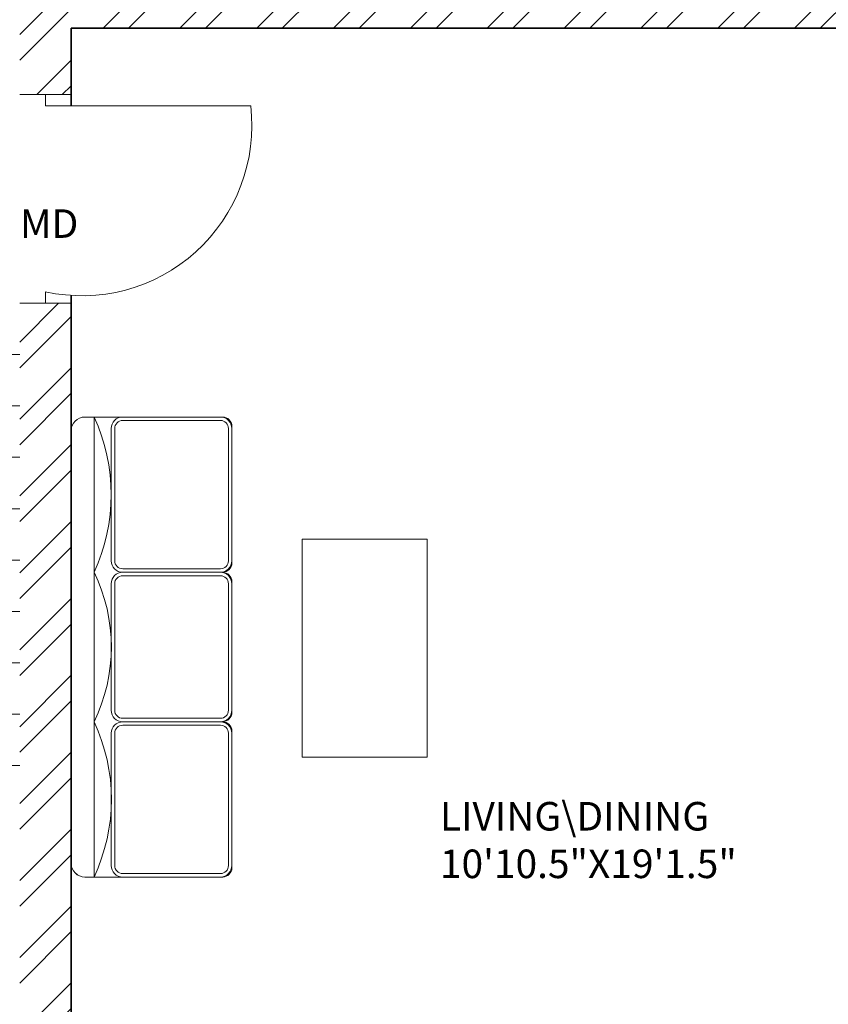
# Model space of a CAD drawing. Units: inches. Extents: x 2120 to 4013, y 1390 to 3019.
# Tile 23 of 59: x 2716 to 2857, y 1792 to 1964. Entities that reach past the tile are written whole.
import ezdxf

# ---------------------------------------------------------------- set-up
doc = ezdxf.new("R2010")
doc.units = ezdxf.units.IN
for name, color, linetype, lineweight in [('A-ANNO-TEXT', 7, 'Continuous', 18), ('A-AREA-IDEN', 7, 'Continuous', 18), ('A-DOOR', 3, 'Continuous', 18), ('A-FLOR-STRS', 7, 'Continuous', 18), ('A-FURN', 8, 'Continuous', 13), ('A-WALL', 7, 'Continuous', 35), ('A-WALL-PATT', 252, 'Continuous', 13)]:
    doc.layers.add(name, color=color, linetype=linetype, lineweight=lineweight)
doc.styles.get("Standard").update_dxf_attribs({"font": 'arial.ttf'})

# ---------------------------------------------------------------- blocks, each defined once
blk = doc.blocks.new('DOOR-SWING-36IN-109p07DEG')
for p, q in [((9, 36.56), (0, 36.56)), ((0, 36.56), (4.5, 36.56)), ((4.5, 36.56), (4.5, 34.56)), ((9, 36.56), (9, 36.56)), ((4.5, 34.56), (40.5, 34.56)), ((4.5, 0), (4.5, 2)), ((9, 0), (0, 0)), ((0, 0), (4.5, 0))]:
    blk.add_line(p, q)
blk.add_arc((10.9, 31.1), 29.8, 257.5927, 6.6652)
blk = doc.blocks.new('TABLE-COFFEE')
blk.add_lwpolyline([(0, 38.19), (21.88, 38.19), (21.88, 0), (0, 0)], close=True)
blk = doc.blocks.new('STAIR-DOGLEG-PLAN')
for p, q in [((60.72, 143.1), (60.72, 31.5)), ((39, 0), (39, 130.5)), ((78, 121.5), (0, 121.5)), ((78, 112.5), (0, 112.5)), ((78, 103.5), (0, 103.5)), ((78, 94.5), (0, 94.5)), ((78, 85.5), (0, 85.5)), ((78, 76.5), (0, 76.5)), ((78, 67.5), (0, 67.5)), ((18.01, 31.5), (18.01, 67.5)), ((78, 58.5), (0, 58.5)), ((78, 49.5), (0, 49.5)), ((60.72, 31.5), (18.01, 31.5)), ((60.72, 31.5), (18.01, 31.5))]:
    blk.add_line(p, q)

msp = doc.modelspace()

# ---------------------------------------------------------------- hatches: boundary and pattern name
at = {"layer": 'A-WALL-PATT'}
h = msp.add_hatch(dxfattribs=at)
h.set_pattern_fill('ANSI32', color=256)
h.paths.add_polyline_path([(2271.7331, 2343.531), (2283.3788, 2343.531), (2283.3788, 2348.031), (2283.3788, 2352.5306), (2262.7331, 2352.5306), (2262.7331, 2182.638), (2267.2331, 2182.638), (2271.7331, 2182.638), (2271.7331, 2219.031), (2391.7331, 2219.031), (2391.7331, 2214.189), (2393.9831, 2214.189), (2396.2331, 2214.189), (2396.2331, 2219.031), (2420.2331, 2219.031), (2420.2331, 2225.7535), (2417.2197, 2225.7535), (2415.7331, 2225.7535), (2415.7331, 2223.5306), (2271.7331, 2223.5306)])
h.paths.add_polyline_path([(2380.0942, 2352.5306), (2343.3788, 2352.5306), (2343.3788, 2343.531), (2363.2331, 2343.531), (2363.2331, 2288.8489), (2365.4831, 2288.8489), (2367.7331, 2288.8489), (2367.7331, 2343.531), (2380.0942, 2343.531)], flags=17)
h.paths.add_polyline_path([(2432.4339, 2352.5306), (2404.0943, 2352.5306), (2404.0943, 2343.531), (2415.7331, 2343.531), (2415.7331, 2264.0306), (2367.7331, 2264.0306), (2367.7331, 2266.4872), (2363.2331, 2266.4872), (2363.2331, 2259.531), (2367.7331, 2259.531), (2415.7331, 2259.531), (2415.7331, 2255.0658), (2420.2331, 2255.0658), (2420.2331, 2259.531), (2424.5717, 2259.531), (2424.5717, 2261.781), (2424.5717, 2264.0306), (2420.2331, 2264.0306), (2420.2331, 2343.531), (2432.4339, 2343.531)])
h.paths.add_polyline_path([(2508.9115, 2352.5306), (2456.4339, 2352.5306), (2456.4339, 2343.531), (2468.2331, 2343.531), (2468.2331, 2264.0306), (2448.0487, 2264.0306), (2448.0487, 2259.531), (2468.2331, 2259.531), (2468.2331, 2255.5496), (2472.7331, 2255.5496), (2472.7331, 2343.531), (2508.9115, 2343.531)])
h.paths.add_polyline_path([(2637.7331, 2352.5306), (2544.9116, 2352.5306), (2544.9116, 2343.531), (2589.7331, 2343.531), (2633.2331, 2343.531), (2637.7331, 2343.531)])
h.paths.add_polyline_path([(2594.2331, 2343.5306), (2589.7331, 2343.5306), (2589.7331, 2259.5306), (2589.7331, 2252.4915), (2591.9831, 2252.4915), (2594.2331, 2252.4915)])
h.paths.add_polyline_path([(2637.7331, 2223.5306), (2594.2331, 2223.5306), (2594.2331, 2230.1988), (2591.9831, 2230.1988), (2589.7331, 2230.1988), (2589.7331, 2223.5306), (2472.7331, 2223.5306), (2468.2331, 2223.5306), (2468.2331, 2219.031), (2628.7331, 2219.031), (2628.7331, 2138.031), (2637.7331, 2138.031)])
h.paths.add_polyline_path([(3822.6535, 2458.4402), (3874.9468, 2458.4402), (3874.9468, 2476.9866), (3822.6535, 2476.9866)], flags=9)
h.paths.add_polyline_path([(3834.6921, 2781.8174), (3935.9206, 2781.8174), (3935.9206, 2800.3638), (3834.6921, 2800.3638)], flags=9)
h.paths.add_polyline_path([(3832.2843, 2837.9683), (3884.5776, 2837.9683), (3884.5776, 2856.5146), (3832.2843, 2856.5146)], flags=9)
h.paths.add_polyline_path([(3830.9388, 2861.4782), (3956.8958, 2861.4782), (3956.8958, 2880.0245), (3830.9388, 2880.0245)], flags=9)
h.paths.add_polyline_path([(3870.6966, 2352.5752), (3887.9272, 2352.5752), (3887.9272, 2377.3037), (3870.6966, 2377.3037)], flags=9)
h.paths.add_polyline_path([(3289.2701, 2413.161), (3435.2223, 2413.161), (3435.2223, 2450.2538), (3289.2701, 2450.2538)], flags=9)
h.paths.add_polyline_path([(2487.6944, 2414.3601), (2637.8335, 2414.3601), (2637.8335, 2451.4528), (2487.6944, 2451.4528)], flags=9)
h.paths.add_polyline_path([(2567.3724, 1457.9199), (2815.296, 1457.9199), (2815.296, 1495.0127), (2567.3724, 1495.0127)], flags=9)
h.paths.add_polyline_path([(2655.3825, 2093.2363), (2685.9555, 2093.2363), (2685.9555, 2111.8937), (2655.3825, 2111.8937)], flags=9)
h.paths.add_polyline_path([(2543.9218, 1550.6671), (2587.8406, 1550.6671), (2587.8406, 1569.3244), (2543.9218, 1569.3244)], flags=9)
h.paths.add_polyline_path([(2905.1384, 1543.8113), (2949.0572, 1543.8113), (2949.0572, 1562.4686), (2905.1384, 1562.4686)], flags=9)
h.paths.add_polyline_path([(2736.4118, 1702.4736), (2784.2153, 1702.4736), (2784.2153, 1721.1309), (2736.4118, 1721.1309)], flags=9)
h.paths.add_polyline_path([(2912.8666, 1710.4168), (2951.707, 1710.4168), (2951.707, 1729.0741), (2912.8666, 1729.0741)], flags=9)
h.paths.add_polyline_path([(2923.5785, 1763.5038), (2959.7279, 1763.5038), (2959.7279, 1782.1611), (2923.5785, 1782.1611)], flags=9)
h.paths.add_polyline_path([(2925.2114, 1809.6137), (2967.1861, 1809.6137), (2967.1861, 1828.271), (2925.2114, 1828.271)], flags=9)
h.paths.add_polyline_path([(2996.2711, 1878.9003), (2996.2711, 1913.109), (2977.6138, 1913.109), (2977.6138, 1878.9003)], flags=9)
h.paths.add_polyline_path([(2883.0859, 1895.7192), (2927.1855, 1895.7192), (2927.1855, 1914.3766), (2883.0859, 1914.3766)], flags=9)
h.paths.add_polyline_path([(2787.3924, 1810.8013), (2841.0213, 1810.8013), (2841.0213, 1829.4587), (2787.3924, 1829.4587)], flags=9)
h.paths.add_polyline_path([(2775.6399, 2101.7395), (2829.2689, 2101.7395), (2829.2689, 2120.3968), (2775.6399, 2120.3968)], flags=9)
h.paths.add_polyline_path([(2913.0263, 2075.817), (2951.8667, 2075.817), (2951.8667, 2094.4744), (2913.0263, 2094.4744)], flags=9)
h.paths.add_polyline_path([(2929.966, 2133.3669), (2966.1154, 2133.3669), (2966.1154, 2152.0243), (2929.966, 2152.0243)], flags=9)
h.paths.add_polyline_path([(2932.7502, 2182.6088), (2968.8996, 2182.6088), (2968.8996, 2201.2662), (2932.7502, 2201.2662)], flags=9)
h.paths.add_polyline_path([(2996.0681, 2266.3173), (2996.0681, 2300.5261), (2977.4108, 2300.5261), (2977.4108, 2266.3173)], flags=9)
h.paths.add_polyline_path([(2885.1039, 2279.2186), (2929.2035, 2279.2186), (2929.2035, 2297.8759), (2885.1039, 2297.8759)], flags=9)
h.paths.add_polyline_path([(2735.7042, 2218.3197), (2783.5078, 2218.3197), (2783.5078, 2236.9771), (2735.7042, 2236.9771)], flags=9)
h.paths.add_polyline_path([(2635.6049, 2044.0085), (2648.9678, 2044.0085), (2648.9678, 2054.312), (2635.6049, 2054.312)], flags=9)
h.paths.add_polyline_path([(2714.0148, 1923.0473), (2727.3777, 1923.0473), (2727.3777, 1933.3508), (2714.0148, 1933.3508)], flags=9)
h.paths.add_polyline_path([(2709.0345, 1988.1628), (2722.3974, 1988.1628), (2722.3974, 1998.4663), (2709.0345, 1998.4663)], flags=9)
h.paths.add_polyline_path([(2592.8935, 1962.1763), (2606.2564, 1962.1763), (2606.2564, 1972.4799), (2592.8935, 1972.4799)], flags=9)
h.paths.add_polyline_path([(2618.3996, 1985.9724), (2644.1942, 1985.9724), (2644.1942, 1996.2759), (2618.3996, 1996.2759)], flags=9)
h.paths.add_polyline_path([(2601.279, 1920.5869), (2614.6419, 1920.5869), (2614.6419, 1930.8904), (2601.279, 1930.8904)], flags=9)
h.paths.add_polyline_path([(2692.3278, 1932.7645), (2704.5311, 1932.7645), (2704.5311, 1943.0681), (2692.3278, 1943.0681)], flags=9)
h.paths.add_polyline_path([(2311.122, 1672.7318), (2355.0408, 1672.7318), (2355.0408, 1691.3892), (2311.122, 1691.3892)], flags=9)
h.paths.add_polyline_path([(2456.2551, 1632.3198), (2492.4796, 1632.3198), (2492.4796, 1650.9772), (2456.2551, 1650.9772)], flags=9)
h.paths.add_polyline_path([(2401.0766, 1631.4793), (2437.301, 1631.4793), (2437.301, 1650.1367), (2401.0766, 1650.1367)], flags=9)
h.paths.add_polyline_path([(2546.7054, 1700.9235), (2594.509, 1700.9235), (2594.509, 1719.5809), (2546.7054, 1719.5809)], flags=9)
h.paths.add_polyline_path([(2445.4866, 1766.9937), (2497.5261, 1766.9937), (2497.5261, 1785.651), (2445.4866, 1785.651)], flags=9)
h.paths.add_polyline_path([(2287.9992, 1739.7675), (2326.8396, 1739.7675), (2326.8396, 1758.4248), (2287.9992, 1758.4248)], flags=9)
h.paths.add_polyline_path([(2458.5279, 1924.7607), (2510.5675, 1924.7607), (2510.5675, 1943.4181), (2458.5279, 1943.4181)], flags=9)
h.paths.add_polyline_path([(2309.2811, 1902.7642), (2345.4305, 1902.7642), (2345.4305, 1921.4215), (2309.2811, 1921.4215)], flags=9)
h.paths.add_polyline_path([(2490.7554, 2018.9392), (2530.7896, 2018.9392), (2530.7896, 2037.5965), (2490.7554, 2037.5965)], flags=9)
h.paths.add_polyline_path([(2402.143, 2024.7393), (2438.5414, 2024.7393), (2438.5414, 2043.3966), (2402.143, 2043.3966)], flags=9)
h.paths.add_polyline_path([(2287.856, 1931.7926), (2326.6964, 1931.7926), (2326.6964, 1950.4499), (2287.856, 1950.4499)], flags=9)
h.paths.add_polyline_path([(2281.7979, 2193.5771), (2320.6383, 2193.5771), (2320.6383, 2212.2344), (2281.7979, 2212.2344)], flags=25)
h.paths.add_polyline_path([(2484.0754, 2093.892), (2536.115, 2093.892), (2536.115, 2112.5494), (2484.0754, 2112.5494)], flags=9)
h.paths.add_polyline_path([(2624.7948, 2281.8639), (2624.7948, 2311.4137), (2606.1375, 2311.4137), (2606.1375, 2281.8639)], flags=9)
h.paths.add_polyline_path([(2507.5036, 2290.3639), (2541.934, 2290.3639), (2541.934, 2309.0212), (2507.5036, 2309.0212)], flags=9)
h.paths.add_polyline_path([(2423.1076, 2285.2202), (2459.332, 2285.2202), (2459.332, 2303.8776), (2423.1076, 2303.8776)], flags=9)
h.paths.add_polyline_path([(2374.5467, 2289.6272), (2410.7711, 2289.6272), (2410.7711, 2308.2846), (2374.5467, 2308.2846)], flags=25)
h.paths.add_polyline_path([(2277.4907, 2227.5651), (2316.3311, 2227.5651), (2316.3311, 2246.2224), (2277.4907, 2246.2224)], flags=25)
h.paths.add_polyline_path([(2655.3825, 2093.2367), (2685.9555, 2093.2367), (2685.9555, 2111.894), (2655.3825, 2111.894)], flags=9)
h.paths.add_polyline_path([(2543.9217, 1550.6674), (2587.8406, 1550.6674), (2587.8406, 1569.3247), (2543.9217, 1569.3247)], flags=9)
h.paths.add_polyline_path([(2905.1384, 1543.8116), (2949.0572, 1543.8116), (2949.0572, 1562.4689), (2905.1384, 1562.4689)], flags=9)
h.paths.add_polyline_path([(2736.4118, 1702.4739), (2784.2153, 1702.4739), (2784.2153, 1721.1312), (2736.4118, 1721.1312)], flags=9)
h.paths.add_polyline_path([(2912.8666, 1710.4171), (2951.707, 1710.4171), (2951.707, 1729.0744), (2912.8666, 1729.0744)], flags=9)
h.paths.add_polyline_path([(2923.5785, 1763.5041), (2959.7279, 1763.5041), (2959.7279, 1782.1614), (2923.5785, 1782.1614)], flags=9)
h.paths.add_polyline_path([(2925.2114, 1809.614), (2967.1861, 1809.614), (2967.1861, 1828.2713), (2925.2114, 1828.2713)], flags=9)
h.paths.add_polyline_path([(2996.2711, 1878.9006), (2996.2711, 1913.1094), (2977.6137, 1913.1094), (2977.6137, 1878.9006)], flags=9)
h.paths.add_polyline_path([(2883.0859, 1895.7195), (2927.1855, 1895.7195), (2927.1855, 1914.3769), (2883.0859, 1914.3769)], flags=9)
h.paths.add_polyline_path([(2787.3924, 1810.8016), (2841.0213, 1810.8016), (2841.0213, 1829.459), (2787.3924, 1829.459)], flags=9)
h.paths.add_polyline_path([(2775.6399, 2101.7398), (2829.2688, 2101.7398), (2829.2688, 2120.3971), (2775.6399, 2120.3971)], flags=9)
h.paths.add_polyline_path([(2913.0263, 2075.8173), (2951.8667, 2075.8173), (2951.8667, 2094.4747), (2913.0263, 2094.4747)], flags=9)
h.paths.add_polyline_path([(2929.966, 2133.3672), (2966.1154, 2133.3672), (2966.1154, 2152.0246), (2929.966, 2152.0246)], flags=9)
h.paths.add_polyline_path([(2932.7502, 2182.6091), (2968.8996, 2182.6091), (2968.8996, 2201.2665), (2932.7502, 2201.2665)], flags=9)
h.paths.add_polyline_path([(2996.0681, 2266.3176), (2996.0681, 2300.5264), (2977.4108, 2300.5264), (2977.4108, 2266.3176)], flags=9)
h.paths.add_polyline_path([(2885.1039, 2279.2189), (2929.2035, 2279.2189), (2929.2035, 2297.8762), (2885.1039, 2297.8762)], flags=9)
h.paths.add_polyline_path([(2735.7042, 2218.32), (2783.5078, 2218.32), (2783.5078, 2236.9774), (2735.7042, 2236.9774)], flags=9)
h.paths.add_polyline_path([(2635.6048, 2044.0088), (2648.9677, 2044.0088), (2648.9677, 2054.3123), (2635.6048, 2054.3123)], flags=9)
h.paths.add_polyline_path([(2714.0148, 1923.0476), (2727.3777, 1923.0476), (2727.3777, 1933.3511), (2714.0148, 1933.3511)], flags=9)
h.paths.add_polyline_path([(2709.0345, 1988.1631), (2722.3974, 1988.1631), (2722.3974, 1998.4666), (2709.0345, 1998.4666)], flags=9)
h.paths.add_polyline_path([(2592.8935, 1962.1766), (2606.2564, 1962.1766), (2606.2564, 1972.4802), (2592.8935, 1972.4802)], flags=9)
h.paths.add_polyline_path([(2618.3995, 1985.9727), (2644.1942, 1985.9727), (2644.1942, 1996.2762), (2618.3995, 1996.2762)], flags=9)
h.paths.add_polyline_path([(2601.279, 1920.5872), (2614.6419, 1920.5872), (2614.6419, 1930.8908), (2601.279, 1930.8908)], flags=9)
h.paths.add_polyline_path([(2692.3278, 1932.7648), (2704.5311, 1932.7648), (2704.5311, 1943.0684), (2692.3278, 1943.0684)], flags=9)
h.paths.add_polyline_path([(2311.122, 1672.7321), (2355.0408, 1672.7321), (2355.0408, 1691.3895), (2311.122, 1691.3895)], flags=9)
h.paths.add_polyline_path([(2456.2551, 1632.3201), (2492.4795, 1632.3201), (2492.4795, 1650.9775), (2456.2551, 1650.9775)], flags=9)
h.paths.add_polyline_path([(2401.0766, 1631.4796), (2437.301, 1631.4796), (2437.301, 1650.137), (2401.0766, 1650.137)], flags=9)
h.paths.add_polyline_path([(2546.7054, 1700.9238), (2594.509, 1700.9238), (2594.509, 1719.5812), (2546.7054, 1719.5812)], flags=9)
h.paths.add_polyline_path([(2445.4866, 1766.994), (2497.5261, 1766.994), (2497.5261, 1785.6513), (2445.4866, 1785.6513)], flags=9)
h.paths.add_polyline_path([(2287.9992, 1739.7678), (2326.8396, 1739.7678), (2326.8396, 1758.4251), (2287.9992, 1758.4251)], flags=9)
h.paths.add_polyline_path([(2458.5279, 1924.7611), (2510.5675, 1924.7611), (2510.5675, 1943.4184), (2458.5279, 1943.4184)], flags=9)
h.paths.add_polyline_path([(2309.2811, 1902.7645), (2345.4305, 1902.7645), (2345.4305, 1921.4218), (2309.2811, 1921.4218)], flags=9)
h.paths.add_polyline_path([(2490.7554, 2018.9395), (2530.7895, 2018.9395), (2530.7895, 2037.5968), (2490.7554, 2037.5968)], flags=9)
h.paths.add_polyline_path([(2402.143, 2024.7396), (2438.5413, 2024.7396), (2438.5413, 2043.3969), (2402.143, 2043.3969)], flags=9)
h.paths.add_polyline_path([(2287.856, 1931.7929), (2326.6964, 1931.7929), (2326.6964, 1950.4502), (2287.856, 1950.4502)], flags=9)
h.paths.add_polyline_path([(2281.7979, 2193.5774), (2320.6383, 2193.5774), (2320.6383, 2212.2347), (2281.7979, 2212.2347)], flags=25)
h.paths.add_polyline_path([(2484.0754, 2093.8924), (2536.115, 2093.8924), (2536.115, 2112.5497), (2484.0754, 2112.5497)], flags=9)
h.paths.add_polyline_path([(2624.7948, 2281.8642), (2624.7948, 2311.414), (2606.1374, 2311.414), (2606.1374, 2281.8642)], flags=9)
h.paths.add_polyline_path([(2507.5035, 2290.3642), (2541.934, 2290.3642), (2541.934, 2309.0215), (2507.5035, 2309.0215)], flags=9)
h.paths.add_polyline_path([(2423.1075, 2285.2205), (2459.332, 2285.2205), (2459.332, 2303.8779), (2423.1075, 2303.8779)], flags=9)
h.paths.add_polyline_path([(2374.5467, 2289.6275), (2410.7711, 2289.6275), (2410.7711, 2308.2849), (2374.5467, 2308.2849)], flags=25)
h.paths.add_polyline_path([(2277.4907, 2227.5654), (2316.3311, 2227.5654), (2316.3311, 2246.2227), (2277.4907, 2246.2227)], flags=25)
h = msp.add_hatch(dxfattribs=at)
h.set_pattern_fill('ANSI32', color=256)
h.paths.add_polyline_path([(2271.7331, 1980.389), (2262.7331, 1980.389), (2262.7331, 1912.8434), (2267.2331, 1912.8434), (2271.7331, 1912.8434), (2271.7331, 1922.531), (2351.2331, 1922.531), (2351.2331, 1901.4728), (2355.7331, 1901.4728), (2355.7331, 1922.531), (2357.9815, 1922.531), (2357.9815, 1926.5306), (2271.7331, 1926.5306)])
h.paths.add_polyline_path([(2589.2331, 1949.1622), (2584.7331, 1949.1622), (2580.2331, 1949.1622), (2580.2331, 1874.5306), (2355.7331, 1874.5306), (2355.7331, 1880.1922), (2351.2331, 1880.1922), (2351.2331, 1874.5306), (2271.7331, 1874.5306), (2271.7331, 1888.8431), (2262.7331, 1888.8431), (2262.7331, 1842.2909), (2267.2331, 1842.2909), (2271.7331, 1842.2909), (2271.7331, 1865.531), (2415.7331, 1865.531), (2415.7331, 1779.7286), (2420.2331, 1779.7286), (2420.2331, 1865.531), (2589.2331, 1865.531)])
h.paths.add_polyline_path([(2271.7331, 1782.2906), (2262.7331, 1782.2906), (2262.7331, 1711.4639), (2267.2331, 1711.4639), (2271.7331, 1711.4639), (2271.7331, 1738.031), (2420.2331, 1738.031), (2420.2331, 1742.531), (2420.2331, 1747.3376), (2417.9831, 1747.3376), (2415.7331, 1747.3376), (2415.7331, 1742.5306), (2271.7331, 1742.5306)])
h.paths.add_polyline_path([(2271.7331, 1627.031), (2362.3957, 1627.031), (2362.3957, 1629.281), (2362.3957, 1631.5306), (2271.7331, 1631.5306), (2271.7331, 1675.4636), (2262.7331, 1675.4636), (2262.7331, 1581.531), (2405.3032, 1581.531), (2405.3032, 1586.031), (2405.3032, 1590.5306), (2396.2331, 1590.5306), (2396.2331, 1691.4513), (2418.7206, 1691.4513), (2418.7206, 1695.951), (2396.2331, 1695.951), (2391.7331, 1695.951), (2391.7331, 1631.5306), (2386.7425, 1631.5306), (2386.7425, 1629.2806), (2386.7425, 1627.031), (2391.7331, 1627.031), (2391.7331, 1586.1709), (2271.7331, 1586.1709)])
h.paths.add_polyline_path([(2459.6703, 1590.5306), (2429.3032, 1590.5306), (2429.3032, 1581.531), (2459.6703, 1581.531), (2459.6703, 1586.031)])
h.paths.add_polyline_path([(2501.2331, 1590.531), (2501.2331, 1665.0195), (2498.9831, 1665.0195), (2496.7331, 1665.0195), (2496.7331, 1590.5306), (2483.8201, 1590.5306), (2483.8201, 1590.1579), (2483.6704, 1590.1579), (2483.6704, 1581.531), (2505.0196, 1581.531), (2505.0196, 1583.781), (2505.0196, 1586.0306), (2501.2331, 1586.0306)])
h.paths.add_polyline_path([(2544.1361, 1583.781), (2544.1361, 1586.0306), (2527.1368, 1586.0306), (2527.1368, 1583.7806), (2527.1368, 1581.531), (2544.1361, 1581.531)])
h.paths.add_polyline_path([(3822.6535, 2458.4402), (3874.9468, 2458.4402), (3874.9468, 2476.9866), (3822.6535, 2476.9866)], flags=9)
h.paths.add_polyline_path([(3834.6921, 2781.8174), (3935.9206, 2781.8174), (3935.9206, 2800.3638), (3834.6921, 2800.3638)], flags=9)
h.paths.add_polyline_path([(3832.2843, 2837.9683), (3884.5776, 2837.9683), (3884.5776, 2856.5146), (3832.2843, 2856.5146)], flags=9)
h.paths.add_polyline_path([(3830.9388, 2861.4782), (3956.8958, 2861.4782), (3956.8958, 2880.0245), (3830.9388, 2880.0245)], flags=9)
h.paths.add_polyline_path([(3870.6966, 2352.5752), (3887.9272, 2352.5752), (3887.9272, 2377.3037), (3870.6966, 2377.3037)], flags=9)
h.paths.add_polyline_path([(3289.2701, 2413.161), (3435.2223, 2413.161), (3435.2223, 2450.2538), (3289.2701, 2450.2538)], flags=9)
h.paths.add_polyline_path([(2487.6944, 2414.3601), (2637.8335, 2414.3601), (2637.8335, 2451.4528), (2487.6944, 2451.4528)], flags=9)
h.paths.add_polyline_path([(2567.3724, 1457.9199), (2815.296, 1457.9199), (2815.296, 1495.0127), (2567.3724, 1495.0127)], flags=9)
h.paths.add_polyline_path([(2655.3825, 2093.2363), (2685.9555, 2093.2363), (2685.9555, 2111.8937), (2655.3825, 2111.8937)], flags=9)
h.paths.add_polyline_path([(2543.9218, 1550.6671), (2587.8406, 1550.6671), (2587.8406, 1569.3244), (2543.9218, 1569.3244)], flags=9)
h.paths.add_polyline_path([(2905.1384, 1543.8113), (2949.0572, 1543.8113), (2949.0572, 1562.4686), (2905.1384, 1562.4686)], flags=9)
h.paths.add_polyline_path([(2736.4118, 1702.4736), (2784.2153, 1702.4736), (2784.2153, 1721.1309), (2736.4118, 1721.1309)], flags=9)
h.paths.add_polyline_path([(2912.8666, 1710.4168), (2951.707, 1710.4168), (2951.707, 1729.0741), (2912.8666, 1729.0741)], flags=9)
h.paths.add_polyline_path([(2923.5785, 1763.5038), (2959.7279, 1763.5038), (2959.7279, 1782.1611), (2923.5785, 1782.1611)], flags=9)
h.paths.add_polyline_path([(2925.2114, 1809.6137), (2967.1861, 1809.6137), (2967.1861, 1828.271), (2925.2114, 1828.271)], flags=9)
h.paths.add_polyline_path([(2996.2711, 1878.9003), (2996.2711, 1913.109), (2977.6138, 1913.109), (2977.6138, 1878.9003)], flags=9)
h.paths.add_polyline_path([(2883.0859, 1895.7192), (2927.1855, 1895.7192), (2927.1855, 1914.3766), (2883.0859, 1914.3766)], flags=9)
h.paths.add_polyline_path([(2787.3924, 1810.8013), (2841.0213, 1810.8013), (2841.0213, 1829.4587), (2787.3924, 1829.4587)], flags=9)
h.paths.add_polyline_path([(2775.6399, 2101.7395), (2829.2689, 2101.7395), (2829.2689, 2120.3968), (2775.6399, 2120.3968)], flags=9)
h.paths.add_polyline_path([(2913.0263, 2075.817), (2951.8667, 2075.817), (2951.8667, 2094.4744), (2913.0263, 2094.4744)], flags=9)
h.paths.add_polyline_path([(2929.966, 2133.3669), (2966.1154, 2133.3669), (2966.1154, 2152.0243), (2929.966, 2152.0243)], flags=9)
h.paths.add_polyline_path([(2932.7502, 2182.6088), (2968.8996, 2182.6088), (2968.8996, 2201.2662), (2932.7502, 2201.2662)], flags=9)
h.paths.add_polyline_path([(2996.0681, 2266.3173), (2996.0681, 2300.5261), (2977.4108, 2300.5261), (2977.4108, 2266.3173)], flags=9)
h.paths.add_polyline_path([(2885.1039, 2279.2186), (2929.2035, 2279.2186), (2929.2035, 2297.8759), (2885.1039, 2297.8759)], flags=9)
h.paths.add_polyline_path([(2735.7042, 2218.3197), (2783.5078, 2218.3197), (2783.5078, 2236.9771), (2735.7042, 2236.9771)], flags=9)
h.paths.add_polyline_path([(2635.6049, 2044.0085), (2648.9678, 2044.0085), (2648.9678, 2054.312), (2635.6049, 2054.312)], flags=9)
h.paths.add_polyline_path([(2714.0148, 1923.0473), (2727.3777, 1923.0473), (2727.3777, 1933.3508), (2714.0148, 1933.3508)], flags=9)
h.paths.add_polyline_path([(2709.0345, 1988.1628), (2722.3974, 1988.1628), (2722.3974, 1998.4663), (2709.0345, 1998.4663)], flags=9)
h.paths.add_polyline_path([(2592.8935, 1962.1763), (2606.2564, 1962.1763), (2606.2564, 1972.4799), (2592.8935, 1972.4799)], flags=9)
h.paths.add_polyline_path([(2618.3996, 1985.9724), (2644.1942, 1985.9724), (2644.1942, 1996.2759), (2618.3996, 1996.2759)], flags=9)
h.paths.add_polyline_path([(2601.279, 1920.5869), (2614.6419, 1920.5869), (2614.6419, 1930.8904), (2601.279, 1930.8904)], flags=9)
h.paths.add_polyline_path([(2692.3278, 1932.7645), (2704.5311, 1932.7645), (2704.5311, 1943.0681), (2692.3278, 1943.0681)], flags=9)
h.paths.add_polyline_path([(2311.122, 1672.7318), (2355.0408, 1672.7318), (2355.0408, 1691.3892), (2311.122, 1691.3892)], flags=25)
h.paths.add_polyline_path([(2456.2551, 1632.3198), (2492.4796, 1632.3198), (2492.4796, 1650.9772), (2456.2551, 1650.9772)], flags=9)
h.paths.add_polyline_path([(2401.0766, 1631.4793), (2437.301, 1631.4793), (2437.301, 1650.1367), (2401.0766, 1650.1367)], flags=9)
h.paths.add_polyline_path([(2546.7054, 1700.9235), (2594.509, 1700.9235), (2594.509, 1719.5809), (2546.7054, 1719.5809)], flags=9)
h.paths.add_polyline_path([(2445.4866, 1766.9937), (2497.5261, 1766.9937), (2497.5261, 1785.651), (2445.4866, 1785.651)], flags=9)
h.paths.add_polyline_path([(2287.9992, 1739.7675), (2326.8396, 1739.7675), (2326.8396, 1758.4248), (2287.9992, 1758.4248)], flags=24)
h.paths.add_polyline_path([(2458.5279, 1924.7607), (2510.5675, 1924.7607), (2510.5675, 1943.4181), (2458.5279, 1943.4181)], flags=25)
h.paths.add_polyline_path([(2309.2811, 1902.7642), (2345.4305, 1902.7642), (2345.4305, 1921.4215), (2309.2811, 1921.4215)], flags=25)
h.paths.add_polyline_path([(2490.7554, 2018.9392), (2530.7896, 2018.9392), (2530.7896, 2037.5965), (2490.7554, 2037.5965)], flags=9)
h.paths.add_polyline_path([(2402.143, 2024.7393), (2438.5414, 2024.7393), (2438.5414, 2043.3966), (2402.143, 2043.3966)], flags=9)
h.paths.add_polyline_path([(2287.856, 1931.7926), (2326.6964, 1931.7926), (2326.6964, 1950.4499), (2287.856, 1950.4499)], flags=25)
h.paths.add_polyline_path([(2281.7979, 2193.5771), (2320.6383, 2193.5771), (2320.6383, 2212.2344), (2281.7979, 2212.2344)], flags=9)
h.paths.add_polyline_path([(2484.0754, 2093.892), (2536.115, 2093.892), (2536.115, 2112.5494), (2484.0754, 2112.5494)], flags=9)
h.paths.add_polyline_path([(2624.7948, 2281.8639), (2624.7948, 2311.4137), (2606.1375, 2311.4137), (2606.1375, 2281.8639)], flags=9)
h.paths.add_polyline_path([(2507.5036, 2290.3639), (2541.934, 2290.3639), (2541.934, 2309.0212), (2507.5036, 2309.0212)], flags=9)
h.paths.add_polyline_path([(2423.1076, 2285.2202), (2459.332, 2285.2202), (2459.332, 2303.8776), (2423.1076, 2303.8776)], flags=9)
h.paths.add_polyline_path([(2374.5467, 2289.6272), (2410.7711, 2289.6272), (2410.7711, 2308.2846), (2374.5467, 2308.2846)], flags=9)
h.paths.add_polyline_path([(2277.4907, 2227.5651), (2316.3311, 2227.5651), (2316.3311, 2246.2224), (2277.4907, 2246.2224)], flags=9)
h.paths.add_polyline_path([(2655.3825, 2093.2367), (2685.9555, 2093.2367), (2685.9555, 2111.894), (2655.3825, 2111.894)], flags=9)
h.paths.add_polyline_path([(2543.9217, 1550.6674), (2587.8406, 1550.6674), (2587.8406, 1569.3247), (2543.9217, 1569.3247)], flags=9)
h.paths.add_polyline_path([(2905.1384, 1543.8116), (2949.0572, 1543.8116), (2949.0572, 1562.4689), (2905.1384, 1562.4689)], flags=9)
h.paths.add_polyline_path([(2736.4118, 1702.4739), (2784.2153, 1702.4739), (2784.2153, 1721.1312), (2736.4118, 1721.1312)], flags=9)
h.paths.add_polyline_path([(2912.8666, 1710.4171), (2951.707, 1710.4171), (2951.707, 1729.0744), (2912.8666, 1729.0744)], flags=9)
h.paths.add_polyline_path([(2923.5785, 1763.5041), (2959.7279, 1763.5041), (2959.7279, 1782.1614), (2923.5785, 1782.1614)], flags=9)
h.paths.add_polyline_path([(2925.2114, 1809.614), (2967.1861, 1809.614), (2967.1861, 1828.2713), (2925.2114, 1828.2713)], flags=9)
h.paths.add_polyline_path([(2996.2711, 1878.9006), (2996.2711, 1913.1094), (2977.6137, 1913.1094), (2977.6137, 1878.9006)], flags=9)
h.paths.add_polyline_path([(2883.0859, 1895.7195), (2927.1855, 1895.7195), (2927.1855, 1914.3769), (2883.0859, 1914.3769)], flags=9)
h.paths.add_polyline_path([(2787.3924, 1810.8016), (2841.0213, 1810.8016), (2841.0213, 1829.459), (2787.3924, 1829.459)], flags=9)
h.paths.add_polyline_path([(2775.6399, 2101.7398), (2829.2688, 2101.7398), (2829.2688, 2120.3971), (2775.6399, 2120.3971)], flags=9)
h.paths.add_polyline_path([(2913.0263, 2075.8173), (2951.8667, 2075.8173), (2951.8667, 2094.4747), (2913.0263, 2094.4747)], flags=9)
h.paths.add_polyline_path([(2929.966, 2133.3672), (2966.1154, 2133.3672), (2966.1154, 2152.0246), (2929.966, 2152.0246)], flags=9)
h.paths.add_polyline_path([(2932.7502, 2182.6091), (2968.8996, 2182.6091), (2968.8996, 2201.2665), (2932.7502, 2201.2665)], flags=9)
h.paths.add_polyline_path([(2996.0681, 2266.3176), (2996.0681, 2300.5264), (2977.4108, 2300.5264), (2977.4108, 2266.3176)], flags=9)
h.paths.add_polyline_path([(2885.1039, 2279.2189), (2929.2035, 2279.2189), (2929.2035, 2297.8762), (2885.1039, 2297.8762)], flags=9)
h.paths.add_polyline_path([(2735.7042, 2218.32), (2783.5078, 2218.32), (2783.5078, 2236.9774), (2735.7042, 2236.9774)], flags=9)
h.paths.add_polyline_path([(2635.6048, 2044.0088), (2648.9677, 2044.0088), (2648.9677, 2054.3123), (2635.6048, 2054.3123)], flags=9)
h.paths.add_polyline_path([(2714.0148, 1923.0476), (2727.3777, 1923.0476), (2727.3777, 1933.3511), (2714.0148, 1933.3511)], flags=9)
h.paths.add_polyline_path([(2709.0345, 1988.1631), (2722.3974, 1988.1631), (2722.3974, 1998.4666), (2709.0345, 1998.4666)], flags=9)
h.paths.add_polyline_path([(2592.8935, 1962.1766), (2606.2564, 1962.1766), (2606.2564, 1972.4802), (2592.8935, 1972.4802)], flags=9)
h.paths.add_polyline_path([(2618.3995, 1985.9727), (2644.1942, 1985.9727), (2644.1942, 1996.2762), (2618.3995, 1996.2762)], flags=9)
h.paths.add_polyline_path([(2601.279, 1920.5872), (2614.6419, 1920.5872), (2614.6419, 1930.8908), (2601.279, 1930.8908)], flags=9)
h.paths.add_polyline_path([(2692.3278, 1932.7648), (2704.5311, 1932.7648), (2704.5311, 1943.0684), (2692.3278, 1943.0684)], flags=9)
h.paths.add_polyline_path([(2311.122, 1672.7321), (2355.0408, 1672.7321), (2355.0408, 1691.3895), (2311.122, 1691.3895)], flags=25)
h.paths.add_polyline_path([(2456.2551, 1632.3201), (2492.4795, 1632.3201), (2492.4795, 1650.9775), (2456.2551, 1650.9775)], flags=9)
h.paths.add_polyline_path([(2401.0766, 1631.4796), (2437.301, 1631.4796), (2437.301, 1650.137), (2401.0766, 1650.137)], flags=9)
h.paths.add_polyline_path([(2546.7054, 1700.9238), (2594.509, 1700.9238), (2594.509, 1719.5812), (2546.7054, 1719.5812)], flags=9)
h.paths.add_polyline_path([(2445.4866, 1766.994), (2497.5261, 1766.994), (2497.5261, 1785.6513), (2445.4866, 1785.6513)], flags=9)
h.paths.add_polyline_path([(2287.9992, 1739.7678), (2326.8396, 1739.7678), (2326.8396, 1758.4251), (2287.9992, 1758.4251)], flags=24)
h.paths.add_polyline_path([(2458.5279, 1924.7611), (2510.5675, 1924.7611), (2510.5675, 1943.4184), (2458.5279, 1943.4184)], flags=25)
h.paths.add_polyline_path([(2309.2811, 1902.7645), (2345.4305, 1902.7645), (2345.4305, 1921.4218), (2309.2811, 1921.4218)], flags=25)
h.paths.add_polyline_path([(2490.7554, 2018.9395), (2530.7895, 2018.9395), (2530.7895, 2037.5968), (2490.7554, 2037.5968)], flags=9)
h.paths.add_polyline_path([(2402.143, 2024.7396), (2438.5413, 2024.7396), (2438.5413, 2043.3969), (2402.143, 2043.3969)], flags=9)
h.paths.add_polyline_path([(2287.856, 1931.7929), (2326.6964, 1931.7929), (2326.6964, 1950.4502), (2287.856, 1950.4502)], flags=25)
h.paths.add_polyline_path([(2281.7979, 2193.5774), (2320.6383, 2193.5774), (2320.6383, 2212.2347), (2281.7979, 2212.2347)], flags=9)
h.paths.add_polyline_path([(2484.0754, 2093.8924), (2536.115, 2093.8924), (2536.115, 2112.5497), (2484.0754, 2112.5497)], flags=9)
h.paths.add_polyline_path([(2624.7948, 2281.8642), (2624.7948, 2311.414), (2606.1374, 2311.414), (2606.1374, 2281.8642)], flags=9)
h.paths.add_polyline_path([(2507.5035, 2290.3642), (2541.934, 2290.3642), (2541.934, 2309.0215), (2507.5035, 2309.0215)], flags=9)
h.paths.add_polyline_path([(2423.1075, 2285.2205), (2459.332, 2285.2205), (2459.332, 2303.8779), (2423.1075, 2303.8779)], flags=9)
h.paths.add_polyline_path([(2374.5467, 2289.6275), (2410.7711, 2289.6275), (2410.7711, 2308.2849), (2374.5467, 2308.2849)], flags=9)
h.paths.add_polyline_path([(2277.4907, 2227.5654), (2316.3311, 2227.5654), (2316.3311, 2246.2227), (2277.4907, 2246.2227)], flags=9)
h = msp.add_hatch(dxfattribs=at)
h.set_pattern_fill('ANSI32', color=256)
h.paths.add_polyline_path([(2271.7331, 2122.6377), (2262.7331, 2122.6377), (2262.7331, 2040.3893), (2267.2331, 2040.3893), (2271.7331, 2040.3893), (2271.7331, 2044.8856), (2271.7331, 2070.531), (2391.7331, 2070.531), (2391.7331, 1926.5306), (2388.3993, 1926.5306), (2388.3993, 1922.531), (2395.7331, 1922.531), (2395.7331, 1992.531), (2400.4511, 1992.531), (2400.4511, 1997.0306), (2395.7331, 1997.0306), (2395.7331, 2070.531), (2443.7331, 2070.531), (2443.7331, 2046.1368), (2448.2331, 2046.1368), (2448.2331, 2070.531), (2580.2331, 2070.531), (2580.2331, 1997.0306), (2492.9076, 1997.0306), (2492.9076, 1992.531), (2580.2331, 1992.531), (2580.2331, 1983.9368), (2589.2331, 1983.9368), (2589.2331, 2070.531), (2589.2331, 2075.0306), (2396.2331, 2075.0306), (2396.2331, 2184.3565), (2393.9831, 2184.3565), (2391.7331, 2184.3565), (2391.7331, 2075.0306), (2271.7331, 2075.0306)])
h.paths.add_polyline_path([(2724.7331, 2138.0306), (2628.7331, 2138.0306), (2628.7331, 2070.5306), (2628.7331, 2067.0987), (2633.2331, 2067.0987), (2637.7331, 2067.0987), (2637.7331, 2070.531), (2657.3413, 2070.531), (2657.3413, 2079.5306), (2637.7331, 2079.5306), (2637.7331, 2129.031), (2715.7331, 2129.031), (2715.7331, 2079.5306), (2698.0378, 2079.5306), (2698.0378, 2070.531), (2715.7331, 2070.531), (2715.7331, 2012.1531), (2720.2331, 2012.1531), (2724.7331, 2012.1531)])
h.paths.add_polyline_path([(2724.7331, 2213.031), (2831.3209, 2213.031), (2831.3209, 2215.281), (2831.3209, 2217.5306), (2724.7331, 2217.5306), (2724.7331, 2343.531), (2751.8755, 2343.531), (2751.8755, 2352.5306), (2715.7331, 2352.5306), (2715.7331, 2138.031), (2724.7331, 2138.031)])
h.paths.add_polyline_path([(2902.53, 2352.5306), (2811.8755, 2352.5306), (2811.8755, 2343.531), (2867.2331, 2343.531), (2867.2331, 2217.5306), (2863.6364, 2217.5306), (2863.6364, 2213.031), (2871.7331, 2213.031), (2871.7331, 2217.531), (2871.7331, 2343.531), (2902.53, 2343.531)])
h.paths.add_polyline_path([(3009.7331, 2352.5306), (2938.53, 2352.5306), (2938.53, 2343.531), (2966.2331, 2343.531), (2966.2331, 2242.3281), (2968.4831, 2242.3281), (2970.7331, 2242.3281), (2970.7331, 2343.531), (3009.7331, 2343.531)])
h.paths.add_polyline_path([(3009.7331, 2217.5306), (2970.7331, 2217.5306), (2970.7331, 2220.5422), (2968.4831, 2220.5422), (2966.2331, 2220.5422), (2966.2331, 2217.5306), (2911.7752, 2217.5306), (2907.7331, 2217.5306), (2907.7331, 2213.0306), (2907.7331, 2194.9663), (2912.2331, 2194.9663), (2912.2331, 2213.031), (2970.7331, 2213.031), (3000.7331, 2213.031), (3000.7331, 2205.523), (3009.7331, 2205.523)])
h.paths.add_polyline_path([(3009.7331, 2181.5227), (3000.7331, 2181.5227), (3000.7331, 2165.0306), (2912.2331, 2165.0306), (2912.2331, 2170.8202), (2907.7331, 2170.8202), (2907.7331, 2165.0306), (2899.5169, 2165.0306), (2899.5169, 2162.7806), (2899.5169, 2160.531), (2907.7331, 2160.531), (2907.7331, 2137.3432), (2912.2331, 2137.3432), (2912.2331, 2160.531), (3000.7331, 2160.531), (3000.7331, 2150.4993), (3009.7331, 2150.4993)])
h.paths.add_polyline_path([(3009.7331, 2126.499), (3005.2331, 2126.499), (3000.7331, 2126.499), (3000.7331, 2112.5306), (2912.2331, 2112.5306), (2912.2331, 2115.6036), (2907.7331, 2115.6036), (2907.7331, 2108.031), (3000.7331, 2108.031), (3000.7331, 2084.7256), (3009.7331, 2084.7256)], flags=17)
h.paths.add_polyline_path([(3009.7331, 1971.531), (3009.7331, 2024.7253), (3000.7331, 2024.7253), (3000.7331, 2006.4153), (3000.7331, 1971.5306), (2864.2331, 1971.5306), (2864.2331, 2160.531), (2868.0522, 2160.531), (2868.0522, 2165.0306), (2859.7331, 2165.0306), (2859.7331, 1971.5306), (2724.7331, 1971.5306), (2724.7331, 1977.7012), (2715.7331, 1977.7012), (2715.7331, 1962.5306), (2715.7331, 1950.9035), (2720.2331, 1950.9035), (2724.7331, 1950.9035), (2724.7331, 1962.531), (2855.2331, 1962.531), (2859.7331, 1962.531), (2859.7331, 1835.031), (2864.2331, 1834.8158), (2864.2331, 1962.531), (2958.7331, 1962.531), (2958.7331, 1937.0925), (2963.2331, 1937.0925), (2963.2331, 1962.531), (3000.7331, 1962.531), (3009.7331, 1962.531)])
h.paths.add_polyline_path([(2724.7331, 1728.531), (2822.7164, 1728.531), (2822.7164, 1733.0306), (2724.7331, 1733.0306), (2724.7331, 1779.3416), (2715.7331, 1779.3416), (2715.7331, 1581.531), (2753.02, 1581.531), (2753.02, 1586.031), (2753.02, 1590.5306), (2724.7331, 1590.5306)])
h.paths.add_polyline_path([(2864.2331, 1590.531), (2864.2331, 1787.031), (2868.4075, 1787.031), (2868.4075, 1791.5306), (2859.7331, 1791.5306), (2859.7331, 1739.0306), (2859.7331, 1733.0306), (2854.3125, 1733.0306), (2854.3125, 1728.531), (2859.7331, 1728.531), (2859.7331, 1590.5306), (2813.02, 1590.5306), (2813.02, 1581.531), (2868.4123, 1581.531), (2868.4123, 1583.781), (2868.4123, 1586.0306), (2864.2331, 1586.0306)])
h.paths.add_polyline_path([(3009.7331, 1754.6619), (3000.7331, 1754.6619), (3000.7331, 1739.0306), (2912.2331, 1739.0306), (2912.2331, 1742.2257), (2907.7331, 1742.2257), (2907.7331, 1739.0306), (2907.7331, 1734.531), (3000.7331, 1734.531), (3000.7331, 1590.5306), (3000.7331, 1586.0306), (2971.3921, 1586.0306), (2971.3921, 1581.531), (3009.7331, 1581.531)])
h.paths.add_polyline_path([(2911.3921, 1583.781), (2911.3921, 1586.0306), (2891.2138, 1586.0306), (2891.2138, 1581.531), (2911.3921, 1581.531)])
h.paths.add_polyline_path([(3009.7331, 1799.8422), (3000.7331, 1799.8422), (3000.7331, 1791.5306), (2912.2331, 1791.5306), (2912.2331, 1796.3264), (2909.9831, 1796.3264), (2907.7331, 1796.3264), (2907.7331, 1791.5306), (2902.7033, 1791.5306), (2902.7033, 1787.031), (2907.7331, 1787.031), (2907.7331, 1761.1622), (2912.2331, 1761.1622), (2912.2331, 1787.031), (3000.7331, 1787.031), (3000.7331, 1778.6622), (3009.7331, 1778.6622)])
h.paths.add_polyline_path([(3009.7331, 1839.5306), (2963.2331, 1839.5306), (2963.2331, 1842.8629), (2960.9831, 1842.8629), (2958.7331, 1842.8629), (2958.7331, 1839.5306), (2907.7331, 1839.5306), (2907.7331, 1814.4599), (2912.2331, 1814.4599), (2912.2331, 1835.031), (3000.7331, 1835.031), (3000.7331, 1823.8425), (3009.7331, 1823.8425), (3009.7331, 1835.031)])
h.paths.add_polyline_path([(2963.2331, 1901.0922), (2960.9831, 1901.0922), (2958.7331, 1901.0922), (2958.7331, 1862.8843), (2963.2331, 1862.8843)], flags=17)
h.paths.add_polyline_path([(2724.7331, 1891.9826), (2724.7331, 1914.3416), (2715.7331, 1914.3416), (2715.7331, 1783.8416), (2637.7331, 1783.8416), (2637.7331, 1914.3416), (2628.7331, 1914.3416), (2624.7701, 1914.3416), (2624.7701, 1909.8416), (2624.7701, 1905.3419), (2628.7331, 1905.3419), (2628.7331, 1876.9915), (2628.7331, 1779.3419), (2637.7331, 1779.3419), (2715.7331, 1779.3419), (2724.7331, 1779.3419), (2724.7331, 1835.031)])
h.paths.add_polyline_path([(2637.7331, 1731.531), (2637.7331, 1779.3416), (2628.7331, 1779.3416), (2628.7331, 1731.5306), (2589.2331, 1731.5306), (2535.9814, 1731.5306), (2496.7331, 1731.5306), (2496.7331, 1725.6876), (2498.9831, 1725.6876), (2501.2331, 1725.6876), (2501.2331, 1727.031), (2628.7331, 1727.031), (2628.7331, 1680.4203), (2628.7331, 1590.5306), (2628.7331, 1586.0306), (2604.1361, 1586.0306), (2604.1361, 1581.531), (2637.7331, 1581.531), (2637.7331, 1590.531)])

# ---------------------------------------------------------------- linework, layer by layer
at = {"layer": 'A-FURN', "ltscale": 0.03}
for points in [[(2752.934, 1868.8374), (2752.934, 1892.7883, 0.41421356), (2751.3225, 1894.3998), (2727.1503, 1894.3998, 0.41421356), (2724.7331, 1891.9826), (2724.7331, 1816.2431, 0.41421356), (2727.1503, 1813.8259), (2751.3225, 1813.8259, 0.41421356), (2752.934, 1815.4374), (2752.934, 1839.3883, 0.41421356), (2751.3225, 1840.9998, -1), (2751.3225, 1841.0394, 0.41421356), (2752.934, 1842.6509), (2752.934, 1865.5748, 0.41421356), (2751.3225, 1867.1863, -1), (2751.3225, 1867.2259, 0.41421356)], [(2752.934, 1868.8371), (2752.934, 1892.788, 0.41421356), (2751.3225, 1894.3995), (2727.1504, 1894.3995, 0.41421356), (2724.7331, 1891.9823), (2724.7331, 1816.2428, 0.41421356), (2727.1504, 1813.8256), (2751.3225, 1813.8256, 0.41421356), (2752.934, 1815.4371), (2752.934, 1839.388, 0.41421356), (2751.3225, 1840.9995, -1), (2751.3225, 1841.0391, 0.41421356), (2752.934, 1842.6506), (2752.934, 1865.5745, 0.41421356), (2751.3225, 1867.186, -1), (2751.3225, 1867.2256, 0.41421356)]]:
    msp.add_lwpolyline(points, format="xyb", close=True, dxfattribs=at)
at = {"layer": 'A-FURN'}
for points in [[(2728.7618, 1894.3998), (2728.7618, 1813.8259)], [(2728.7618, 1894.3995), (2728.7618, 1813.8256)]]:
    msp.add_lwpolyline(points, dxfattribs=at)
for points in [[(2750.9196, 1894.3998), (2733.7977, 1894.3998, 0.41421356), (2731.7833, 1892.3855), (2731.7833, 1869.2205, 0.41421356), (2733.7977, 1867.2061), (2750.9196, 1867.2061, 0.41421356), (2752.934, 1869.2205), (2752.934, 1892.3855, 0.41421356)], [(2750.9197, 1894.3995), (2733.7977, 1894.3995, 0.41421356), (2731.7834, 1892.3852), (2731.7834, 1869.2202, 0.41421356), (2733.7977, 1867.2058), (2750.9197, 1867.2058, 0.41421356), (2752.934, 1869.2202), (2752.934, 1892.3852, 0.41421356)], [(2750.9196, 1893.7955), (2733.7977, 1893.7955, 0.41421356), (2732.3876, 1892.3855), (2732.3876, 1869.2205, 0.41421356), (2733.7977, 1867.8104), (2750.9196, 1867.8104, 0.41421356), (2752.3297, 1869.2205), (2752.3297, 1892.3855, 0.41421356)], [(2750.9197, 1893.7952), (2733.7977, 1893.7952, 0.41421356), (2732.3877, 1892.3852), (2732.3877, 1869.2202, 0.41421356), (2733.7977, 1867.8101), (2750.9197, 1867.8101, 0.41421356), (2752.3297, 1869.2202), (2752.3297, 1892.3852, 0.41421356)], [(2750.9196, 1841.0196), (2733.7977, 1841.0196, -0.41421356), (2731.7833, 1843.0339), (2731.7833, 1865.1918, -0.41421356), (2733.7977, 1867.2061), (2750.9196, 1867.2061, -0.41421356), (2752.934, 1865.1918), (2752.934, 1843.0339, -0.41421356)], [(2750.9197, 1841.0193), (2733.7977, 1841.0193, -0.41421356), (2731.7834, 1843.0336), (2731.7834, 1865.1915, -0.41421356), (2733.7977, 1867.2058), (2750.9197, 1867.2058, -0.41421356), (2752.934, 1865.1915), (2752.934, 1843.0336, -0.41421356)], [(2750.9196, 1841.6239), (2733.7977, 1841.6239, -0.41421356), (2732.3876, 1843.0339), (2732.3876, 1865.1918, -0.41421356), (2733.7977, 1866.6018), (2750.9196, 1866.6018, -0.41421356), (2752.3297, 1865.1918), (2752.3297, 1843.0339, -0.41421356)], [(2750.9197, 1841.6236), (2733.7977, 1841.6236, -0.41421356), (2732.3877, 1843.0336), (2732.3877, 1865.1915, -0.41421356), (2733.7977, 1866.6015), (2750.9197, 1866.6015, -0.41421356), (2752.3297, 1865.1915), (2752.3297, 1843.0336, -0.41421356)], [(2750.9196, 1841.0196), (2733.7977, 1841.0196, 0.41421356), (2731.7833, 1839.0053), (2731.7833, 1815.8403, 0.41421356), (2733.7977, 1813.8259), (2750.9196, 1813.8259, 0.41421356), (2752.934, 1815.8403), (2752.934, 1839.0053, 0.41421356)], [(2750.9197, 1841.0193), (2733.7977, 1841.0193, 0.41421356), (2731.7834, 1839.0049), (2731.7834, 1815.84, 0.41421356), (2733.7977, 1813.8256), (2750.9197, 1813.8256, 0.41421356), (2752.934, 1815.84), (2752.934, 1839.0049, 0.41421356)], [(2750.9196, 1840.4153), (2733.7977, 1840.4153, 0.41421356), (2732.3876, 1839.0053), (2732.3876, 1815.8403, 0.41421356), (2733.7977, 1814.4302), (2750.9196, 1814.4302, 0.41421356), (2752.3297, 1815.8403), (2752.3297, 1839.0053, 0.41421356)], [(2750.9197, 1840.415), (2733.7977, 1840.415, 0.41421356), (2732.3877, 1839.0049), (2732.3877, 1815.84, 0.41421356), (2733.7977, 1814.4299), (2750.9197, 1814.4299, 0.41421356), (2752.3297, 1815.84), (2752.3297, 1839.0049, 0.41421356)]]:
    msp.add_lwpolyline(points, format="xyb", close=True, dxfattribs=at)
for centre, radius, start, end in [((2699.7216, 1880.803), 32.0657, 334.910626, 25.089374), ((2699.7217, 1880.8027), 32.0657, 334.910626, 25.089374), ((2702.0717, 1854.1129), 29.7287, 333.868999, 26.131001), ((2702.0717, 1854.1126), 29.7287, 333.868999, 26.131001), ((2700.0574, 1827.4228), 31.7619, 334.653824, 25.346176), ((2700.0574, 1827.4225), 31.7619, 334.653824, 25.346176)]:
    msp.add_arc(centre, radius, start, end, dxfattribs=at)
at = {"layer": 'A-WALL'}
for p, q in [((2724.7331, 1962.531), (2855.2331, 1962.531)), ((2859.7331, 1962.531), (2724.7331, 1962.531)), ((2724.7331, 1948.9035), (2724.7331, 1962.531)), ((2859.7331, 1962.5306), (2724.7331, 1962.5306)), ((2724.7331, 1948.9032), (2724.7331, 1962.5306)), ((2724.7331, 1962.5306), (2855.2331, 1962.5306)), ((2724.7331, 1839.531), (2724.7331, 1915.7067)), ((2724.7331, 1839.5306), (2724.7331, 1915.7064)), ((2724.7331, 1839.531), (2724.7331, 1835.031)), ((2724.7331, 1839.5306), (2724.7331, 1835.0306)), ((2724.7331, 1733.031), (2724.7331, 1835.031)), ((2724.7331, 1733.0306), (2724.7331, 1835.0306))]:
    msp.add_line(p, q, dxfattribs=at)

# ---------------------------------------------------------------- block references
at = {"layer": 'A-DOOR'}
for p in [(2715.7331, 1914.3419), (2715.7331, 1914.3416)]:
    msp.add_blockref('DOOR-SWING-36IN-109p07DEG', p, dxfattribs=at)
at = {"layer": 'A-FLOR-STRS'}
msp.add_blockref('STAIR-DOGLEG-PLAN', (2637.7331, 1783.8416), dxfattribs=at)
at = {"layer": 'A-FURN'}
for p in [(2765.2578, 1834.8246), (2765.2579, 1834.8243)]:
    msp.add_blockref('TABLE-COFFEE', p, dxfattribs=at)

# ---------------------------------------------------------------- texts
at = {"layer": 'A-ANNO-TEXT', "char_height": 5, "attachment_point": 1}
for insert in [(2715.7832, 1930.7778), (2715.7832, 1930.7775)]:
    msp.add_mtext_dynamic_manual_height_columns('MD', width=56.213303, gutter_width=12.5, heights=[0], dxfattribs=dict(at, insert=insert))
at = {"layer": 'A-AREA-IDEN', "char_height": 5, "attachment_point": 1}
for insert in [(2789.403, 1826.9709), (2789.403, 1826.9706)]:
    msp.add_mtext_dynamic_manual_height_columns('LIVING\\\\DINING\\P10\'10.5"X19\'1.5"', width=321.685562, gutter_width=12.5, heights=[0], dxfattribs=dict(at, insert=insert))

doc.saveas('drawing.dxf')
